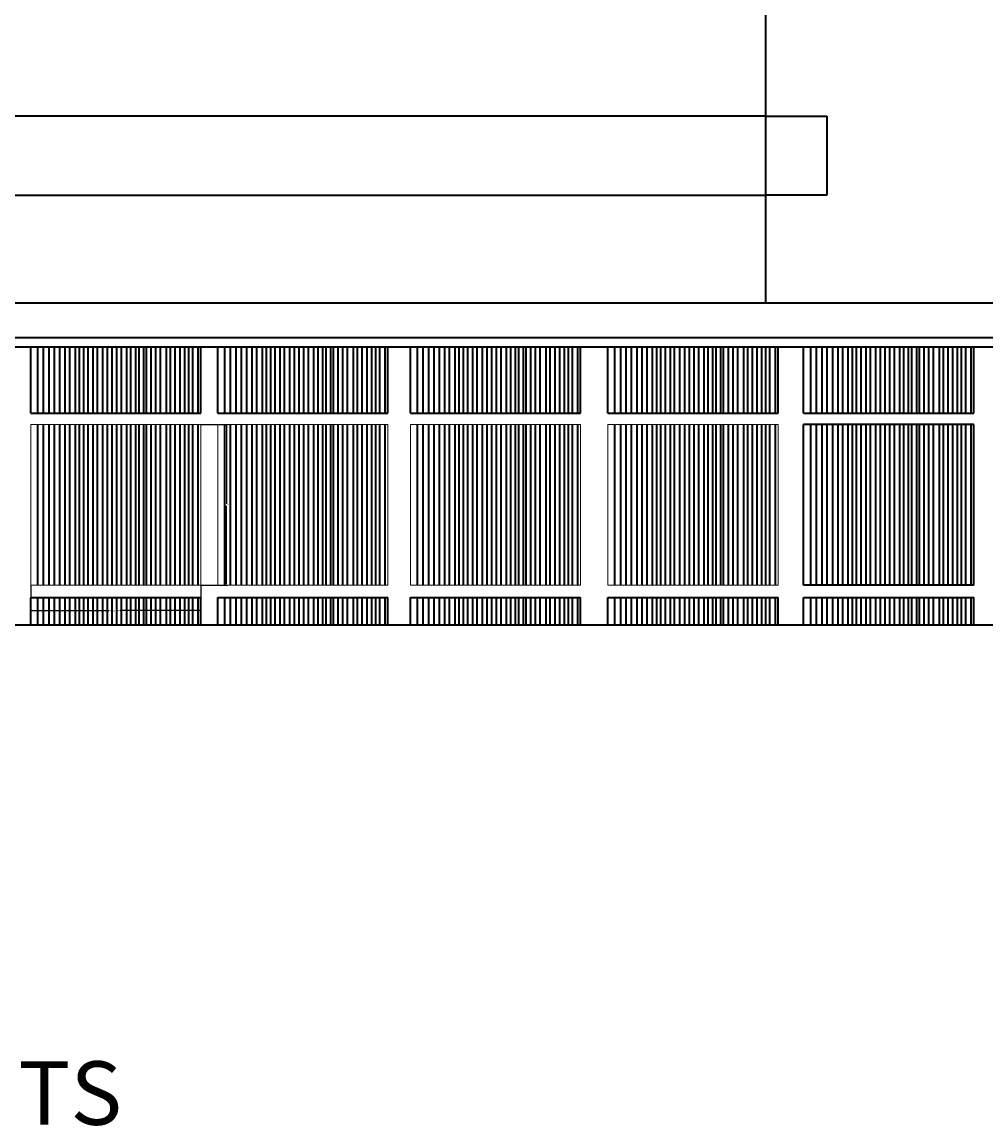
# Model space of a CAD drawing. Units: inches. Extents: x -1080 to 1950, y -1929 to 857.
# Tile 9 of 16: x 1333 to 1495, y -819 to -633. Entities that reach past the tile are written whole.
import ezdxf

# ---------------------------------------------------------------- set-up
doc = ezdxf.new("R2010")
doc.units = ezdxf.units.IN
doc.header["$MEASUREMENT"] = 0
for name, color, linetype, lineweight in [('A-ANNO-DIMS', 2, 'Continuous', 18), ('A-ANNO-TEXT', 7, 'Continuous', 25), ('A-ELEV', 7, 'Continuous', 35), ('A-GLAZ', 4, 'Continuous', 18)]:
    doc.layers.add(name, color=color, linetype=linetype, lineweight=lineweight)
doc.styles.get("Standard").update_dxf_attribs({"font": 'arial.ttf'})
doc.dimstyles.get("Standard").update_dxf_attribs({"dimtxt": 0.18, "dimasz": 0.18, "dimexe": 0.18, "dimexo": 0.0625, "dimgap": 0.09, "dimtad": 0, "dimtih": 1, "dimtoh": 1, "dimdec": 4, "dimzin": 0, "dimdsep": 46, "dimtxsty": 'Standard', "dimcen": 0.09, "dimadec": 0, "dimazin": 0, "dimtfac": 1, "dimtdec": 4, "dimtofl": 0, "dimtmove": 0, "dimatfit": 3, "dimfxl": 1, "dimtolj": 1, "dimtzin": 0, "dimarcsym": 0})

# ---------------------------------------------------------------- blocks, each defined once
blk = doc.blocks.new('PANEL-C')
for p, q in [((0, 0), (0, 27)), ((28.56, 27), (0, 27)), ((28.56, 0), (28.56, 27)), ((28.56, 0), (0, 0))]:
    blk.add_line(p, q)
blk = doc.blocks.new('*D75')
at = {"layer": 'A-ANNO-DIMS', "color": 0, "lineweight": -2, "transparency": 16777216}
for p, q in [((1334.64, -728.13), (1334.64, -732.53)), ((1363.2, -728.13), (1363.2, -732.53)), ((1334.82, -732.35), (1347.82, -732.35)), ((1363.02, -732.35), (1350.01, -732.35))]:
    blk.add_line(p, q, dxfattribs=at)
at = {"layer": 'A-ANNO-DIMS', "color": 0, "transparency": 16777216}
for points in [[(1334.82, -732.32), (1334.82, -732.38), (1334.64, -732.35)], [(1363.02, -732.32), (1363.02, -732.38), (1363.2, -732.35)]]:
    blk.add_solid(points, dxfattribs=at)
at = {"layer": 'Defpoints', "color": 0, "transparency": 16777216}
for p in [(1334.64, -728.07), (1363.2, -728.07), (1363.2, -732.35)]:
    blk.add_point(p, dxfattribs=at)
at = {"layer": 'A-ANNO-DIMS', "color": 0, "transparency": 16777216, "insert": (1348.92, -732.35), "char_height": 0.18, "attachment_point": 5}
blk.add_mtext('\\A1;PANEL C 29 TYP.', dxfattribs=at)
blk = doc.blocks.new('*D76')
at = {"layer": 'A-ANNO-DIMS', "color": 0, "lineweight": -2, "transparency": 16777216}
for p, q in [((1363.26, -701.07), (1367.66, -701.07)), ((1367.48, -701.25), (1367.48, -714.39)), ((1367.48, -727.89), (1367.48, -714.75)), ((1363.26, -728.07), (1367.66, -728.07))]:
    blk.add_line(p, q, dxfattribs=at)
at = {"layer": 'A-ANNO-DIMS', "color": 0, "transparency": 16777216}
for points in [[(1367.45, -701.25), (1367.51, -701.25), (1367.48, -701.07)], [(1367.45, -727.89), (1367.51, -727.89), (1367.48, -728.07)]]:
    blk.add_solid(points, dxfattribs=at)
at = {"layer": 'Defpoints', "color": 0, "transparency": 16777216}
for p in [(1363.2, -701.07), (1367.48, -701.07), (1363.2, -728.07)]:
    blk.add_point(p, dxfattribs=at)
at = {"layer": 'A-ANNO-DIMS', "color": 0, "transparency": 16777216, "insert": (1367.48, -714.57), "char_height": 0.18, "attachment_point": 5}
blk.add_mtext('\\A1;27 TYP.', dxfattribs=at)

msp = doc.modelspace()

# ---------------------------------------------------------------- linework, layer by layer
at = {"layer": 'A-ELEV'}
for p, q in [((1458.07, -680.68), (1458.07, -629.59)), ((1458.07, -649.29), (1120.45, -649.29)), ((1458.07, -649.29), (1468.27, -649.29)), ((1468.27, -649.29), (1468.27, -662.56)), ((1120.45, -662.56), (1458.07, -662.56)), ((1468.27, -662.56), (1458.07, -662.56)), ((1627.86, -680.68), (1123.47, -680.68)), ((1123.47, -686.45), (1622.49, -686.45)), ((1123.47, -688.04), (1622.49, -688.04)), ((1334.64, -699.19), (1334.64, -688.04)), ((1335.83, -699.19), (1335.83, -688.04)), ((1336.8, -699.19), (1336.8, -688.04)), ((1337.73, -699.19), (1337.73, -688.04)), ((1338.61, -699.19), (1338.61, -688.04)), ((1339.53, -699.19), (1339.53, -688.04)), ((1340.41, -699.19), (1340.41, -688.04)), ((1341.2, -699.19), (1341.2, -688.04)), ((1342.13, -699.19), (1342.13, -688.04)), ((1342.83, -699.19), (1342.83, -688.04)), ((1343.54, -699.19), (1343.54, -688.04)), ((1344.29, -699.19), (1344.29, -688.04)), ((1345.12, -699.19), (1345.12, -688.04)), ((1345.84, -699.19), (1345.84, -688.04)), ((1346.74, -699.19), (1346.74, -688.04)), ((1347.53, -699.19), (1347.53, -688.04)), ((1348.32, -699.19), (1348.32, -688.04)), ((1349.11, -699.19), (1349.11, -688.04)), ((1349.9, -699.19), (1349.9, -688.04)), ((1350.8, -699.19), (1350.8, -688.04)), ((1351.47, -699.19), (1351.47, -688.04)), ((1352.26, -699.19), (1352.26, -688.04)), ((1352.83, -699.19), (1352.83, -688.04)), ((1353.62, -699.19), (1353.62, -688.04)), ((1354.07, -699.19), (1354.07, -688.04)), ((1354.86, -699.19), (1354.86, -688.04)), ((1355.64, -699.19), (1355.64, -688.04)), ((1356.43, -699.19), (1356.43, -688.04)), ((1357.45, -699.19), (1357.45, -688.04)), ((1358.12, -699.19), (1358.12, -688.04)), ((1358.91, -699.19), (1358.91, -688.04)), ((1359.7, -699.19), (1359.7, -688.04)), ((1360.49, -699.19), (1360.49, -688.04)), ((1361.17, -699.19), (1361.17, -688.04)), ((1361.84, -699.19), (1361.84, -688.04)), ((1362.75, -699.19), (1362.75, -688.04)), ((1363.2, -699.19), (1363.2, -688.04)), ((1366.03, -699.19), (1366.03, -688.04)), ((1367.23, -699.19), (1367.23, -688.04)), ((1368.2, -699.19), (1368.2, -688.04)), ((1369.12, -699.19), (1369.12, -688.04)), ((1370, -699.19), (1370, -688.04)), ((1370.93, -699.19), (1370.93, -688.04)), ((1371.81, -699.19), (1371.81, -688.04)), ((1372.6, -699.19), (1372.6, -688.04)), ((1373.53, -699.19), (1373.53, -688.04)), ((1374.23, -699.19), (1374.23, -688.04)), ((1374.94, -699.19), (1374.94, -688.04)), ((1375.68, -699.19), (1375.68, -688.04)), ((1376.52, -699.19), (1376.52, -688.04)), ((1377.24, -699.19), (1377.24, -688.04)), ((1378.14, -699.19), (1378.14, -688.04)), ((1378.93, -699.19), (1378.93, -688.04)), ((1379.72, -699.19), (1379.72, -688.04)), ((1380.5, -699.19), (1380.5, -688.04)), ((1381.29, -699.19), (1381.29, -688.04)), ((1382.19, -699.19), (1382.19, -688.04)), ((1382.87, -699.19), (1382.87, -688.04)), ((1383.66, -699.19), (1383.66, -688.04)), ((1384.22, -699.19), (1384.22, -688.04)), ((1385.01, -699.19), (1385.01, -688.04)), ((1385.46, -699.19), (1385.46, -688.04)), ((1386.25, -699.19), (1386.25, -688.04)), ((1387.04, -699.19), (1387.04, -688.04)), ((1387.83, -699.19), (1387.83, -688.04)), ((1388.85, -699.19), (1388.85, -688.04)), ((1389.52, -699.19), (1389.52, -688.04)), ((1390.31, -699.19), (1390.31, -688.04)), ((1391.1, -699.19), (1391.1, -688.04)), ((1391.89, -699.19), (1391.89, -688.04)), ((1392.56, -699.19), (1392.56, -688.04)), ((1393.24, -699.19), (1393.24, -688.04)), ((1394.14, -699.19), (1394.14, -688.04)), ((1394.59, -699.19), (1394.59, -688.04)), ((1398.38, -699.19), (1398.38, -688.04)), ((1399.58, -699.19), (1399.58, -688.04)), ((1400.54, -699.19), (1400.54, -688.04)), ((1401.47, -699.19), (1401.47, -688.04)), ((1402.35, -699.19), (1402.35, -688.04)), ((1403.27, -699.19), (1403.27, -688.04)), ((1404.16, -699.19), (1404.16, -688.04)), ((1404.95, -699.19), (1404.95, -688.04)), ((1405.87, -699.19), (1405.87, -688.04)), ((1406.58, -699.19), (1406.58, -688.04)), ((1407.28, -699.19), (1407.28, -688.04)), ((1408.03, -699.19), (1408.03, -688.04)), ((1408.87, -699.19), (1408.87, -688.04)), ((1409.58, -699.19), (1409.58, -688.04)), ((1410.48, -699.19), (1410.48, -688.04)), ((1411.27, -699.19), (1411.27, -688.04)), ((1412.06, -699.19), (1412.06, -688.04)), ((1412.85, -699.19), (1412.85, -688.04)), ((1413.64, -699.19), (1413.64, -688.04)), ((1414.54, -699.19), (1414.54, -688.04)), ((1415.22, -699.19), (1415.22, -688.04)), ((1416.01, -699.19), (1416.01, -688.04)), ((1416.57, -699.19), (1416.57, -688.04)), ((1417.36, -699.19), (1417.36, -688.04)), ((1417.81, -699.19), (1417.81, -688.04)), ((1418.6, -699.19), (1418.6, -688.04)), ((1419.39, -699.19), (1419.39, -688.04)), ((1420.18, -699.19), (1420.18, -688.04)), ((1421.19, -699.19), (1421.19, -688.04)), ((1421.87, -699.19), (1421.87, -688.04)), ((1422.66, -699.19), (1422.66, -688.04)), ((1423.45, -699.19), (1423.45, -688.04)), ((1424.23, -699.19), (1424.23, -688.04)), ((1424.91, -699.19), (1424.91, -688.04)), ((1425.59, -699.19), (1425.59, -688.04)), ((1426.49, -699.19), (1426.49, -688.04)), ((1426.94, -699.19), (1426.94, -688.04)), ((1431.54, -699.19), (1431.54, -688.04)), ((1432.73, -699.19), (1432.73, -688.04)), ((1433.7, -699.19), (1433.7, -688.04)), ((1434.63, -699.19), (1434.63, -688.04)), ((1435.51, -699.19), (1435.51, -688.04)), ((1436.43, -699.19), (1436.43, -688.04)), ((1437.31, -699.19), (1437.31, -688.04)), ((1438.11, -699.19), (1438.11, -688.04)), ((1439.03, -699.19), (1439.03, -688.04)), ((1439.74, -699.19), (1439.74, -688.04)), ((1440.44, -699.19), (1440.44, -688.04)), ((1441.19, -699.19), (1441.19, -688.04)), ((1442.03, -699.19), (1442.03, -688.04)), ((1442.74, -699.19), (1442.74, -688.04)), ((1443.64, -699.19), (1443.64, -688.04)), ((1444.43, -699.19), (1444.43, -688.04)), ((1445.22, -699.19), (1445.22, -688.04)), ((1446.01, -699.19), (1446.01, -688.04)), ((1446.8, -699.19), (1446.8, -688.04)), ((1447.7, -699.19), (1447.7, -688.04)), ((1448.38, -699.19), (1448.38, -688.04)), ((1449.16, -699.19), (1449.16, -688.04)), ((1449.73, -699.19), (1449.73, -688.04)), ((1450.52, -699.19), (1450.52, -688.04)), ((1450.97, -699.19), (1450.97, -688.04)), ((1451.76, -699.19), (1451.76, -688.04)), ((1452.55, -699.19), (1452.55, -688.04)), ((1453.33, -699.19), (1453.33, -688.04)), ((1454.35, -699.19), (1454.35, -688.04)), ((1455.03, -699.19), (1455.03, -688.04)), ((1455.81, -699.19), (1455.81, -688.04)), ((1456.6, -699.19), (1456.6, -688.04)), ((1457.39, -699.19), (1457.39, -688.04)), ((1458.07, -699.19), (1458.07, -688.04)), ((1458.07, -699.19), (1458.07, -688.04)), ((1458.75, -699.19), (1458.75, -688.04)), ((1459.65, -699.19), (1459.65, -688.04)), ((1460.1, -699.19), (1460.1, -688.04)), ((1464.4, -699.19), (1464.4, -688.04)), ((1465.6, -699.19), (1465.6, -688.04)), ((1466.57, -699.19), (1466.57, -688.04)), ((1467.49, -699.19), (1467.49, -688.04)), ((1468.37, -699.19), (1468.37, -688.04)), ((1469.3, -699.19), (1469.3, -688.04)), ((1470.18, -699.19), (1470.18, -688.04)), ((1470.97, -699.19), (1470.97, -688.04)), ((1471.9, -699.19), (1471.9, -688.04)), ((1472.6, -699.19), (1472.6, -688.04)), ((1473.3, -699.19), (1473.3, -688.04)), ((1474.05, -699.19), (1474.05, -688.04)), ((1474.89, -699.19), (1474.89, -688.04)), ((1475.6, -699.19), (1475.6, -688.04)), ((1476.51, -699.19), (1476.51, -688.04)), ((1477.3, -699.19), (1477.3, -688.04)), ((1478.08, -699.19), (1478.08, -688.04)), ((1478.87, -699.19), (1478.87, -688.04)), ((1479.66, -699.19), (1479.66, -688.04)), ((1480.56, -699.19), (1480.56, -688.04)), ((1481.24, -699.19), (1481.24, -688.04)), ((1482.03, -699.19), (1482.03, -688.04)), ((1482.59, -699.19), (1482.59, -688.04)), ((1483.38, -699.19), (1483.38, -688.04)), ((1483.83, -699.19), (1483.83, -688.04)), ((1484.62, -699.19), (1484.62, -688.04)), ((1485.41, -699.19), (1485.41, -688.04)), ((1486.2, -699.19), (1486.2, -688.04)), ((1487.21, -699.19), (1487.21, -688.04)), ((1487.89, -699.19), (1487.89, -688.04)), ((1488.68, -699.19), (1488.68, -688.04)), ((1489.47, -699.19), (1489.47, -688.04)), ((1490.26, -699.19), (1490.26, -688.04)), ((1490.93, -699.19), (1490.93, -688.04)), ((1491.61, -699.19), (1491.61, -688.04)), ((1492.51, -699.19), (1492.51, -688.04)), ((1492.96, -699.19), (1492.96, -688.04)), ((1334.64, -699.19), (1363.2, -699.19)), ((1366.03, -699.19), (1394.59, -699.19)), ((1398.38, -699.19), (1426.94, -699.19)), ((1431.54, -699.19), (1460.1, -699.19)), ((1464.4, -699.19), (1492.96, -699.19)), ((1335.83, -728.07), (1335.83, -701.07)), ((1336.8, -728.07), (1336.8, -701.07)), ((1337.73, -728.07), (1337.73, -701.07)), ((1338.61, -728.07), (1338.61, -701.07)), ((1339.53, -728.07), (1339.53, -701.07)), ((1340.41, -728.07), (1340.41, -701.07)), ((1341.2, -728.07), (1341.2, -701.07)), ((1342.13, -728.07), (1342.13, -701.07)), ((1342.83, -728.07), (1342.83, -701.07)), ((1343.54, -728.07), (1343.54, -701.07)), ((1344.29, -728.07), (1344.29, -701.07)), ((1345.12, -728.07), (1345.12, -701.07)), ((1345.84, -728.07), (1345.84, -701.07)), ((1346.74, -728.07), (1346.74, -701.07)), ((1347.53, -728.07), (1347.53, -701.07)), ((1348.32, -728.07), (1348.32, -701.07)), ((1349.11, -728.07), (1349.11, -701.07)), ((1349.9, -728.07), (1349.9, -701.07)), ((1350.8, -728.07), (1350.8, -701.07)), ((1351.47, -728.07), (1351.47, -701.07)), ((1352.26, -728.07), (1352.26, -701.07)), ((1352.83, -728.07), (1352.83, -701.07)), ((1353.62, -728.07), (1353.62, -701.07)), ((1354.07, -728.07), (1354.07, -701.07)), ((1354.86, -728.07), (1354.86, -701.07)), ((1355.64, -728.07), (1355.64, -701.07)), ((1356.43, -728.07), (1356.43, -701.07)), ((1357.45, -728.07), (1357.45, -701.07)), ((1358.12, -728.07), (1358.12, -701.07)), ((1358.91, -728.07), (1358.91, -701.07)), ((1359.7, -728.07), (1359.7, -701.07)), ((1360.49, -728.07), (1360.49, -701.07)), ((1361.17, -728.07), (1361.17, -701.07)), ((1361.84, -728.07), (1361.84, -701.07)), ((1362.75, -728.07), (1362.75, -701.07)), ((1367.23, -728.07), (1367.23, -701.07)), ((1368.2, -728.07), (1368.2, -701.07)), ((1369.12, -728.07), (1369.12, -701.07)), ((1370, -728.07), (1370, -701.07)), ((1370.93, -728.07), (1370.93, -701.07)), ((1371.81, -728.07), (1371.81, -701.07)), ((1372.6, -728.07), (1372.6, -701.07)), ((1373.53, -728.07), (1373.53, -701.07)), ((1374.23, -728.07), (1374.23, -701.07)), ((1374.94, -728.07), (1374.94, -701.07)), ((1375.68, -728.07), (1375.68, -701.07)), ((1376.52, -728.07), (1376.52, -701.07)), ((1377.24, -728.07), (1377.24, -701.07)), ((1378.14, -728.07), (1378.14, -701.07)), ((1378.93, -728.07), (1378.93, -701.07)), ((1379.72, -728.07), (1379.72, -701.07)), ((1380.5, -728.07), (1380.5, -701.07)), ((1381.29, -728.07), (1381.29, -701.07)), ((1382.19, -728.07), (1382.19, -701.07)), ((1382.87, -728.07), (1382.87, -701.07)), ((1383.66, -728.07), (1383.66, -701.07)), ((1384.22, -728.07), (1384.22, -701.07)), ((1385.01, -728.07), (1385.01, -701.07)), ((1385.46, -728.07), (1385.46, -701.07)), ((1386.25, -728.07), (1386.25, -701.07)), ((1387.04, -728.07), (1387.04, -701.07)), ((1387.83, -728.07), (1387.83, -701.07)), ((1388.85, -728.07), (1388.85, -701.07)), ((1389.52, -728.07), (1389.52, -701.07)), ((1390.31, -728.07), (1390.31, -701.07)), ((1391.1, -728.07), (1391.1, -701.07)), ((1391.89, -728.07), (1391.89, -701.07)), ((1392.56, -728.07), (1392.56, -701.07)), ((1393.24, -728.07), (1393.24, -701.07)), ((1394.14, -728.07), (1394.14, -701.07)), ((1399.58, -728.07), (1399.58, -701.07)), ((1400.54, -728.07), (1400.54, -701.07)), ((1401.47, -728.07), (1401.47, -701.07)), ((1402.35, -728.07), (1402.35, -701.07)), ((1403.27, -728.07), (1403.27, -701.07)), ((1404.16, -728.07), (1404.16, -701.07)), ((1404.95, -728.07), (1404.95, -701.07)), ((1405.87, -728.07), (1405.87, -701.07)), ((1406.58, -728.07), (1406.58, -701.07)), ((1407.28, -728.07), (1407.28, -701.07)), ((1408.03, -728.07), (1408.03, -701.07)), ((1408.87, -728.07), (1408.87, -701.07)), ((1409.58, -728.07), (1409.58, -701.07)), ((1410.48, -728.07), (1410.48, -701.07)), ((1411.27, -728.07), (1411.27, -701.07)), ((1412.06, -728.07), (1412.06, -701.07)), ((1412.85, -728.07), (1412.85, -701.07)), ((1413.64, -728.07), (1413.64, -701.07)), ((1414.54, -728.07), (1414.54, -701.07)), ((1415.22, -728.07), (1415.22, -701.07)), ((1416.01, -728.07), (1416.01, -701.07)), ((1416.57, -728.07), (1416.57, -701.07)), ((1417.36, -728.07), (1417.36, -701.07)), ((1417.81, -728.07), (1417.81, -701.07)), ((1418.6, -728.07), (1418.6, -701.07)), ((1419.39, -728.07), (1419.39, -701.07)), ((1420.18, -728.07), (1420.18, -701.07)), ((1421.19, -728.07), (1421.19, -701.07)), ((1421.87, -728.07), (1421.87, -701.07)), ((1422.66, -728.07), (1422.66, -701.07)), ((1423.45, -728.07), (1423.45, -701.07)), ((1424.23, -728.07), (1424.23, -701.07)), ((1424.91, -728.07), (1424.91, -701.07)), ((1425.59, -728.07), (1425.59, -701.07)), ((1426.49, -728.07), (1426.49, -701.07)), ((1432.73, -728.07), (1432.73, -701.07)), ((1433.7, -728.07), (1433.7, -701.07)), ((1434.63, -728.07), (1434.63, -701.07)), ((1435.51, -728.07), (1435.51, -701.07)), ((1436.43, -728.07), (1436.43, -701.07)), ((1437.31, -728.07), (1437.31, -701.07)), ((1438.11, -728.07), (1438.11, -701.07)), ((1439.03, -728.07), (1439.03, -701.07)), ((1439.74, -728.07), (1439.74, -701.07)), ((1440.44, -728.07), (1440.44, -701.07)), ((1441.19, -728.07), (1441.19, -701.07)), ((1442.03, -728.07), (1442.03, -701.07)), ((1442.74, -728.07), (1442.74, -701.07)), ((1443.64, -728.07), (1443.64, -701.07)), ((1444.43, -728.07), (1444.43, -701.07)), ((1445.22, -728.07), (1445.22, -701.07)), ((1446.01, -728.07), (1446.01, -701.07)), ((1446.8, -728.07), (1446.8, -701.07)), ((1447.7, -728.07), (1447.7, -701.07)), ((1448.38, -728.07), (1448.38, -701.07)), ((1449.16, -728.07), (1449.16, -701.07)), ((1449.73, -728.07), (1449.73, -701.07)), ((1450.52, -728.07), (1450.52, -701.07)), ((1450.97, -728.07), (1450.97, -701.07)), ((1451.76, -728.07), (1451.76, -701.07)), ((1452.55, -728.07), (1452.55, -701.07)), ((1453.33, -728.07), (1453.33, -701.07)), ((1454.35, -728.07), (1454.35, -701.07)), ((1455.03, -728.07), (1455.03, -701.07)), ((1455.81, -728.07), (1455.81, -701.07)), ((1456.6, -728.07), (1456.6, -701.07)), ((1457.39, -728.07), (1457.39, -701.07)), ((1458.07, -728.07), (1458.07, -701.07)), ((1458.07, -728.07), (1458.07, -701.07)), ((1458.75, -728.07), (1458.75, -701.07)), ((1459.65, -728.07), (1459.65, -701.07)), ((1464.4, -728.07), (1464.4, -701.07)), ((1492.96, -701.07), (1464.4, -701.07)), ((1465.6, -728.07), (1465.6, -701.07)), ((1466.57, -728.07), (1466.57, -701.07)), ((1467.49, -728.07), (1467.49, -701.07)), ((1468.37, -728.07), (1468.37, -701.07)), ((1469.3, -728.07), (1469.3, -701.07)), ((1470.18, -728.07), (1470.18, -701.07)), ((1470.97, -728.07), (1470.97, -701.07)), ((1471.9, -728.07), (1471.9, -701.07)), ((1472.6, -728.07), (1472.6, -701.07)), ((1473.3, -728.07), (1473.3, -701.07)), ((1474.05, -728.07), (1474.05, -701.07)), ((1474.89, -728.07), (1474.89, -701.07)), ((1475.6, -728.07), (1475.6, -701.07)), ((1476.51, -728.07), (1476.51, -701.07)), ((1477.3, -728.07), (1477.3, -701.07)), ((1478.08, -728.07), (1478.08, -701.07)), ((1478.87, -728.07), (1478.87, -701.07)), ((1479.66, -728.07), (1479.66, -701.07)), ((1480.56, -728.07), (1480.56, -701.07)), ((1481.24, -728.07), (1481.24, -701.07)), ((1482.03, -728.07), (1482.03, -701.07)), ((1482.59, -728.07), (1482.59, -701.07)), ((1483.38, -728.07), (1483.38, -701.07)), ((1483.83, -728.07), (1483.83, -701.07)), ((1484.62, -728.07), (1484.62, -701.07)), ((1485.41, -728.07), (1485.41, -701.07)), ((1486.2, -728.07), (1486.2, -701.07)), ((1487.21, -728.07), (1487.21, -701.07)), ((1487.89, -728.07), (1487.89, -701.07)), ((1488.68, -728.07), (1488.68, -701.07)), ((1489.47, -728.07), (1489.47, -701.07)), ((1490.26, -728.07), (1490.26, -701.07)), ((1490.93, -728.07), (1490.93, -701.07)), ((1491.61, -728.07), (1491.61, -701.07)), ((1492.51, -728.07), (1492.51, -701.07)), ((1492.96, -728.07), (1492.96, -701.07)), ((1492.96, -728.07), (1464.4, -728.07)), ((1334.64, -734.72), (1334.64, -730.16)), ((1334.64, -730.16), (1363.2, -730.16)), ((1335.83, -734.72), (1335.83, -730.16)), ((1336.8, -734.72), (1336.8, -730.16)), ((1337.73, -734.72), (1337.73, -730.16)), ((1338.61, -734.72), (1338.61, -730.16)), ((1339.53, -734.72), (1339.53, -730.16)), ((1340.41, -734.72), (1340.41, -730.16)), ((1341.2, -734.72), (1341.2, -730.16)), ((1342.13, -734.72), (1342.13, -730.16)), ((1342.83, -734.72), (1342.83, -730.16)), ((1343.54, -734.72), (1343.54, -730.16)), ((1344.29, -734.72), (1344.29, -730.16)), ((1345.12, -734.72), (1345.12, -730.16)), ((1345.84, -734.72), (1345.84, -730.16)), ((1346.74, -734.72), (1346.74, -730.16)), ((1347.53, -734.72), (1347.53, -730.16)), ((1348.32, -734.72), (1348.32, -730.16)), ((1349.11, -734.72), (1349.11, -730.16)), ((1349.9, -734.72), (1349.9, -730.16)), ((1350.8, -734.72), (1350.8, -730.16)), ((1351.47, -734.72), (1351.47, -730.16)), ((1352.26, -734.72), (1352.26, -730.16)), ((1352.83, -734.72), (1352.83, -730.16)), ((1353.62, -734.72), (1353.62, -730.16)), ((1354.07, -734.72), (1354.07, -730.16)), ((1354.86, -734.72), (1354.86, -730.16)), ((1355.64, -734.72), (1355.64, -730.16)), ((1356.43, -734.72), (1356.43, -730.16)), ((1357.45, -734.72), (1357.45, -730.16)), ((1358.12, -734.72), (1358.12, -730.16)), ((1358.91, -734.72), (1358.91, -730.16)), ((1359.7, -734.72), (1359.7, -730.16)), ((1360.49, -734.72), (1360.49, -730.16)), ((1361.17, -734.72), (1361.17, -730.16)), ((1361.84, -734.72), (1361.84, -730.16)), ((1362.75, -734.72), (1362.75, -730.16)), ((1363.2, -734.72), (1363.2, -730.16)), ((1366.03, -734.72), (1366.03, -730.16)), ((1366.03, -730.16), (1394.59, -730.16)), ((1367.23, -734.72), (1367.23, -730.16)), ((1368.2, -734.72), (1368.2, -730.16)), ((1369.12, -734.72), (1369.12, -730.16)), ((1370, -734.72), (1370, -730.16)), ((1370.93, -734.72), (1370.93, -730.16)), ((1371.81, -734.72), (1371.81, -730.16)), ((1372.6, -734.72), (1372.6, -730.16)), ((1373.53, -734.72), (1373.53, -730.16)), ((1374.23, -734.72), (1374.23, -730.16)), ((1374.94, -734.72), (1374.94, -730.16)), ((1375.68, -734.72), (1375.68, -730.16)), ((1376.52, -734.72), (1376.52, -730.16)), ((1377.24, -734.72), (1377.24, -730.16)), ((1378.14, -734.72), (1378.14, -730.16)), ((1378.93, -734.72), (1378.93, -730.16)), ((1379.72, -734.72), (1379.72, -730.16)), ((1380.5, -734.72), (1380.5, -730.16)), ((1381.29, -734.72), (1381.29, -730.16)), ((1382.19, -734.72), (1382.19, -730.16)), ((1382.87, -734.72), (1382.87, -730.16)), ((1383.66, -734.72), (1383.66, -730.16)), ((1384.22, -734.72), (1384.22, -730.16)), ((1385.01, -734.72), (1385.01, -730.16)), ((1385.46, -734.72), (1385.46, -730.16)), ((1386.25, -734.72), (1386.25, -730.16)), ((1387.04, -734.72), (1387.04, -730.16)), ((1387.83, -734.72), (1387.83, -730.16)), ((1388.85, -734.72), (1388.85, -730.16)), ((1389.52, -734.72), (1389.52, -730.16)), ((1390.31, -734.72), (1390.31, -730.16)), ((1391.1, -734.72), (1391.1, -730.16)), ((1391.89, -734.72), (1391.89, -730.16)), ((1392.56, -734.72), (1392.56, -730.16)), ((1393.24, -734.72), (1393.24, -730.16)), ((1394.14, -734.72), (1394.14, -730.16)), ((1394.59, -734.72), (1394.59, -730.16)), ((1398.38, -734.72), (1398.38, -730.16)), ((1398.38, -730.16), (1426.94, -730.16)), ((1399.58, -734.72), (1399.58, -730.16)), ((1400.54, -734.72), (1400.54, -730.16)), ((1401.47, -734.72), (1401.47, -730.16)), ((1402.35, -734.72), (1402.35, -730.16)), ((1403.27, -734.72), (1403.27, -730.16)), ((1404.16, -734.72), (1404.16, -730.16)), ((1404.95, -734.72), (1404.95, -730.16)), ((1405.87, -734.72), (1405.87, -730.16)), ((1406.58, -734.72), (1406.58, -730.16)), ((1407.28, -734.72), (1407.28, -730.16)), ((1408.03, -734.72), (1408.03, -730.16)), ((1408.87, -734.72), (1408.87, -730.16)), ((1409.58, -734.72), (1409.58, -730.16)), ((1410.48, -734.72), (1410.48, -730.16)), ((1411.27, -734.72), (1411.27, -730.16)), ((1412.06, -734.72), (1412.06, -730.16)), ((1412.85, -734.72), (1412.85, -730.16)), ((1413.64, -734.72), (1413.64, -730.16)), ((1414.54, -734.72), (1414.54, -730.16)), ((1415.22, -734.72), (1415.22, -730.16)), ((1416.01, -734.72), (1416.01, -730.16)), ((1416.57, -734.72), (1416.57, -730.16)), ((1417.36, -734.72), (1417.36, -730.16)), ((1417.81, -734.72), (1417.81, -730.16)), ((1418.6, -734.72), (1418.6, -730.16)), ((1419.39, -734.72), (1419.39, -730.16)), ((1420.18, -734.72), (1420.18, -730.16)), ((1421.19, -734.72), (1421.19, -730.16)), ((1421.87, -734.72), (1421.87, -730.16)), ((1422.66, -734.72), (1422.66, -730.16)), ((1423.45, -734.72), (1423.45, -730.16)), ((1424.23, -734.72), (1424.23, -730.16)), ((1424.91, -734.72), (1424.91, -730.16)), ((1425.59, -734.72), (1425.59, -730.16)), ((1426.49, -734.72), (1426.49, -730.16)), ((1426.94, -734.72), (1426.94, -730.16)), ((1431.54, -734.72), (1431.54, -730.16)), ((1431.54, -730.16), (1460.1, -730.16)), ((1432.73, -734.72), (1432.73, -730.16)), ((1433.7, -734.72), (1433.7, -730.16)), ((1434.63, -734.72), (1434.63, -730.16)), ((1435.51, -734.72), (1435.51, -730.16)), ((1436.43, -734.72), (1436.43, -730.16)), ((1437.31, -734.72), (1437.31, -730.16)), ((1438.11, -734.72), (1438.11, -730.16)), ((1439.03, -734.72), (1439.03, -730.16)), ((1439.74, -734.72), (1439.74, -730.16)), ((1440.44, -734.72), (1440.44, -730.16)), ((1441.19, -734.72), (1441.19, -730.16)), ((1442.03, -734.72), (1442.03, -730.16)), ((1442.74, -734.72), (1442.74, -730.16)), ((1443.64, -734.72), (1443.64, -730.16)), ((1444.43, -734.72), (1444.43, -730.16)), ((1445.22, -734.72), (1445.22, -730.16)), ((1446.01, -734.72), (1446.01, -730.16)), ((1446.8, -734.72), (1446.8, -730.16)), ((1447.7, -734.72), (1447.7, -730.16)), ((1448.38, -734.72), (1448.38, -730.16)), ((1449.16, -734.72), (1449.16, -730.16)), ((1449.73, -734.72), (1449.73, -730.16)), ((1450.52, -734.72), (1450.52, -730.16)), ((1450.97, -734.72), (1450.97, -730.16)), ((1451.76, -734.72), (1451.76, -730.16)), ((1452.55, -734.72), (1452.55, -730.16)), ((1453.33, -734.72), (1453.33, -730.16)), ((1454.35, -734.72), (1454.35, -730.16)), ((1455.03, -734.72), (1455.03, -730.16)), ((1455.81, -734.72), (1455.81, -730.16)), ((1456.6, -734.72), (1456.6, -730.16)), ((1457.39, -734.72), (1457.39, -730.16)), ((1458.07, -734.72), (1458.07, -730.16)), ((1458.07, -734.72), (1458.07, -730.16)), ((1458.75, -734.72), (1458.75, -730.16)), ((1459.65, -734.72), (1459.65, -730.16)), ((1460.1, -734.72), (1460.1, -730.16)), ((1464.4, -734.72), (1464.4, -730.16)), ((1464.4, -730.16), (1492.96, -730.16)), ((1465.6, -734.72), (1465.6, -730.16)), ((1466.57, -734.72), (1466.57, -730.16)), ((1467.49, -734.72), (1467.49, -730.16)), ((1468.37, -734.72), (1468.37, -730.16)), ((1469.3, -734.72), (1469.3, -730.16)), ((1470.18, -734.72), (1470.18, -730.16)), ((1470.97, -734.72), (1470.97, -730.16)), ((1471.9, -734.72), (1471.9, -730.16)), ((1472.6, -734.72), (1472.6, -730.16)), ((1473.3, -734.72), (1473.3, -730.16)), ((1474.05, -734.72), (1474.05, -730.16)), ((1474.89, -734.72), (1474.89, -730.16)), ((1475.6, -734.72), (1475.6, -730.16)), ((1476.51, -734.72), (1476.51, -730.16)), ((1477.3, -734.72), (1477.3, -730.16)), ((1478.08, -734.72), (1478.08, -730.16)), ((1478.87, -734.72), (1478.87, -730.16)), ((1479.66, -734.72), (1479.66, -730.16)), ((1480.56, -734.72), (1480.56, -730.16)), ((1481.24, -734.72), (1481.24, -730.16)), ((1482.03, -734.72), (1482.03, -730.16)), ((1482.59, -734.72), (1482.59, -730.16)), ((1483.38, -734.72), (1483.38, -730.16)), ((1483.83, -734.72), (1483.83, -730.16)), ((1484.62, -734.72), (1484.62, -730.16)), ((1485.41, -734.72), (1485.41, -730.16)), ((1486.2, -734.72), (1486.2, -730.16)), ((1487.21, -734.72), (1487.21, -730.16)), ((1487.89, -734.72), (1487.89, -730.16)), ((1488.68, -734.72), (1488.68, -730.16)), ((1489.47, -734.72), (1489.47, -730.16)), ((1490.26, -734.72), (1490.26, -730.16)), ((1490.93, -734.72), (1490.93, -730.16)), ((1491.61, -734.72), (1491.61, -730.16)), ((1492.51, -734.72), (1492.51, -730.16)), ((1492.96, -734.72), (1492.96, -730.16)), ((998.14, -734.72), (1442.74, -734.72)), ((1442.74, -734.72), (1691.4, -734.72))]:
    msp.add_line(p, q, dxfattribs=at)

# ---------------------------------------------------------------- block references
at = {"layer": 'A-GLAZ'}
for p in [(1334.64, -728.07), (1366.03, -728.07), (1398.38, -728.07), (1431.54, -728.07)]:
    msp.add_blockref('PANEL-C', p, dxfattribs=at)

# ---------------------------------------------------------------- texts
at = {"layer": 'A-ANNO-TEXT'}
msp.add_text('MAINTENANCE   ACCESS   POINTS', height=10.6643, dxfattribs=at).set_placement((1124.46, -818.72))

# ---------------------------------------------------------------- dimensions: what is measured, and where the dimension line sits
at = {"layer": 'A-ANNO-DIMS'}
dim = msp.add_linear_dim(base=(1367.48, -701.07), p1=(1363.2, -728.07), p2=(1363.2, -701.07), angle=90, text='<> TYP.', dimstyle='Standard', override={"dimdec": 0, "dimlfac": 1, "dimrnd": 0, "dimzin": 0, "dimdsep": 46, "dimlunit": 2}, dxfattribs=at)
dim.commit()
dim.dimension.update_dxf_attribs({"geometry": '*D76', "text_midpoint": (1367.48, -714.57)})
dim = msp.add_linear_dim(base=(1363.2, -732.35), p1=(1334.64, -728.07), p2=(1363.2, -728.07), text='PANEL C <> TYP.', dimstyle='Standard', override={"dimdec": 0, "dimlfac": 1, "dimrnd": 0, "dimzin": 0, "dimdsep": 46, "dimlunit": 2}, dxfattribs=at)
dim.commit()
dim.dimension.update_dxf_attribs({"geometry": '*D75', "text_midpoint": (1348.92, -732.35)})

doc.saveas('drawing.dxf')
